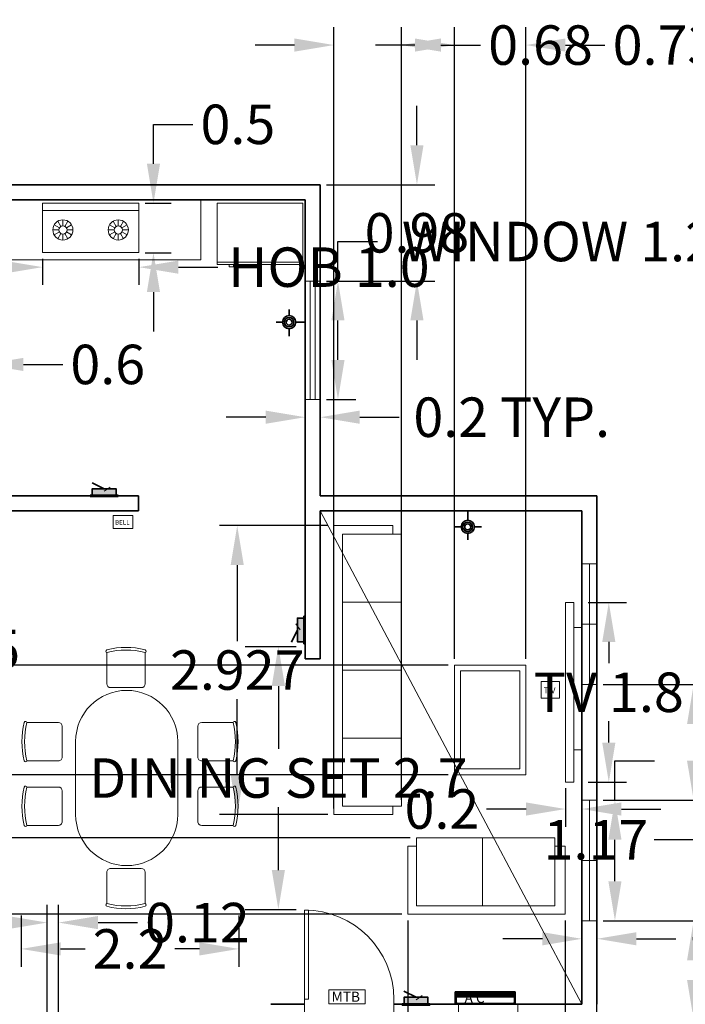
# Model space of a CAD drawing. Units: metres. Extents: x 24.2 to 58.5, y -14.5 to 15.2.
# Tile 6 of 7: x 45.2 to 51.9, y 5.2 to 15.2. Entities that reach past the tile are written whole.
import ezdxf

# ---------------------------------------------------------------- set-up
doc = ezdxf.new("R2010")
doc.units = ezdxf.units.M
doc.header["$MEASUREMENT"] = 0
for name, color, linetype, lineweight in [('A-EQPM', 163, 'Continuous', 18), ('A-FLOR', 7, 'Continuous', 25), ('A-FLOR-CASE', 163, 'Continuous', 18), ('A-GLAZ', 15, 'Continuous', 18), ('A-WALL', 7, 'Continuous', 35), ('DIMENSION', 90, 'Continuous', 18), ('DOOR', 15, 'Continuous', 18), ('E-COMM', 1, 'Continuous', 18), ('E-EQPM-LAYO', 1, 'Continuous', 13), ('E-LITE', 1, 'Continuous', 18), ('E-POWR', 1, 'Continuous', 18), ('E-POWR-EQPM', 1, 'Continuous', 18), ('Elec', 1, 'Continuous', 35), ('FURN', 163, 'Continuous', 13)]:
    doc.layers.add(name, color=color, linetype=linetype, lineweight=lineweight)
doc.styles.get("Standard").update_dxf_attribs({"font": 'arial.ttf'})
doc.dimstyles.get("Standard").update_dxf_attribs({"dimtxt": 0.4, "dimasz": 0.4, "dimexe": 0.18, "dimexo": 0.0625, "dimgap": 0.09, "dimtad": 0, "dimtih": 1, "dimtoh": 1, "dimdec": 1, "dimzin": 0, "dimdsep": 46, "dimtxsty": 'Standard', "dimcen": 0.09, "dimadec": 0, "dimazin": 0, "dimtfac": 1, "dimtdec": 1, "dimtofl": 0, "dimtmove": 0, "dimatfit": 3, "dimfxl": 1, "dimtolj": 1, "dimtzin": 0, "dimarcsym": 0})

# ---------------------------------------------------------------- blocks, each defined once
blk = doc.blocks.new('*U17')
for p, q in [((0, 0), (0, -6)), ((40, 0), (40, -6))]:
    blk.add_line(p, q)
blk.add_lwpolyline([(0, 0), (0, 40), (1.75, 40), (1.75, 0)], close=True)
blk.add_arc((0, 0), 40, 0, 90)
blk = doc.blocks.new('TV')
for points in [[(1846.64, 1133.16), (1849.49, 1133.16), (1849.49, 1073.14), (1846.64, 1073.14)], [(1846.64, 1122.37), (1844, 1122.37), (1844, 1081.48), (1846.64, 1081.48)]]:
    blk.add_lwpolyline(points, close=True)
blk = doc.blocks.new('DCHARRND')
for p, q in [((-10, -2.63815), (-10, -18.99995)), ((10, -18.99995), (10, -2.63815)), ((-8, -20.99995), (8, -20.99995))]:
    blk.add_line(p, q)
for centre, radius, start, end in [((0, -41.272), 41.272, 75.97797, 104.022), ((-9.7697, -1.94695), 0.75323, 107.8005, 188.662), ((-9.8649, -2.00005), 0.65223, 185.3119, 258.05), ((0, -42.68032), 41.272, 75.97797, 104.022), ((9.7697, -1.94695), 0.75323, 351.338, 72.19953), ((9.865, -2.00005), 0.65223, 281.95, 354.6881), ((-8, -18.99995), 2, 180, 270), ((8, -18.99995), 2, 270, 0)]:
    blk.add_arc(centre, radius, start, end)
blk = doc.blocks.new('TABLE')
for p, q in [((59.132, -4.604), (59.132, -5.611)), ((60.539, -4.604), (60.539, -5.611))]:
    blk.add_line(p, q)
for centre, start, end in [((59.836, -4.604), 0, 180), ((59.836, -5.611), 180, 0)]:
    blk.add_arc(centre, 0.704, start, end)
at = {"layer": 'FURN', "xscale": -0.0264381201488454, "yscale": 0.0264381201488454, "zscale": 0.0264381201488454}
blk.add_blockref('DCHARRND', (59.826, -3.307), dxfattribs=at)
at = {"layer": 'FURN', "yscale": 0.0264381201488454, "zscale": 0.0264381201488454}
for p, xscale, rotation in [((58.391, -4.606), -0.0264381201488454, 89.99999999999991), ((61.372, -4.606), 0.0264381201488454, 270.0000000000001), ((58.391, -5.496), -0.0264381201488454, 89.99999999999991), ((61.372, -5.496), 0.0264381201488454, 270.0000000000001), ((59.826, -6.908), 0.0264381201488454, 180)]:
    blk.add_blockref('DCHARRND', p, dxfattribs=dict(at, xscale=xscale, rotation=rotation))
blk = doc.blocks.new('*U31')
blk.add_line((0, 1), (0, -1))
blk = doc.blocks.new('*U32')
at = {"layer": 'FURN', "transparency": 16777216}
for p, rotation in [((1740.24, 1059.29), 30), ((1742.61, 1059.29), 330.0000000000001), ((1739.06, 1057.24), 90), ((1739.38, 1058.42), 59.99999999999999), ((1739.38, 1056.06), 120), ((1743.47, 1058.42), 300), ((1743.47, 1056.06), 240), ((1743.79, 1057.24), 270), ((1740.24, 1055.19), 150), ((1741.42, 1054.87), 180), ((1742.61, 1055.19), 210)]:
    blk.add_blockref('*U31', p, dxfattribs=dict(at, rotation=rotation))
blk.add_blockref('*U31', (1741.42, 1059.61), dxfattribs=at)
blk = doc.blocks.new('*U33')
blk.add_line((0, 1), (0, -1))
blk = doc.blocks.new('*U34')
at = {"layer": 'FURN', "transparency": 16777216}
for p, rotation in [((1740.24, 1059.29), 30), ((1742.61, 1059.29), 330.0000000000001), ((1739.06, 1057.24), 90), ((1739.38, 1058.42), 59.99999999999999), ((1739.38, 1056.06), 120), ((1743.47, 1058.42), 300), ((1743.47, 1056.06), 240), ((1743.79, 1057.24), 270), ((1740.24, 1055.19), 150), ((1741.42, 1054.87), 180), ((1742.61, 1055.19), 210)]:
    blk.add_blockref('*U33', p, dxfattribs=dict(at, rotation=rotation))
blk.add_blockref('*U33', (1741.42, 1059.61), dxfattribs=at)
blk = doc.blocks.new('GAS')
at = {"layer": 'FURN'}
blk.add_line((1734.58, 1063.74), (1766.85, 1063.74), dxfattribs=at)
blk.add_lwpolyline([(1734.58, 1066.15), (1766.85, 1066.15), (1766.85, 1049.65), (1734.58, 1049.65)], close=True, dxfattribs=at)
for centre, radius in [((1741.42, 1057.24), 3.37), ((1759.93, 1057.24), 3.37), ((1741.42, 1057.24), 1.37), ((1759.93, 1057.24), 1.37)]:
    blk.add_circle(centre, radius, dxfattribs=at)
for name, p in [('*U32', (0, 0)), ('*U34', (18.51, 0))]:
    blk.add_blockref(name, p, dxfattribs=at)
blk = doc.blocks.new('splight')
at = {"layer": 'Elec'}
for p, q in [((4618.17, 527.16), (4627.57, 527.16)), ((4622.87, 527.16), (4622.87, 523.87)), ((4620.58, 521.58), (4618.05, 521.58)), ((4625.16, 521.58), (4627.23, 521.58)), ((4622.87, 519.28), (4622.87, 517.03))]:
    blk.add_line(p, q, dxfattribs=at)
for radius in [2.29, 1.67, 1.04]:
    blk.add_circle((4622.87, 521.58), radius, dxfattribs=at)
blk = doc.blocks.new('WINDOW-1200')
for p, q in [((0.1529, 1.1998), (0.0005, 1.1998)), ((0.0513, -0.0002), (0.0513, 1.1998)), ((0.1021, -0.0002), (0.1021, 1.1998)), ((0.1529, -0.0002), (0.0005, -0.0002))]:
    blk.add_line(p, q)
blk = doc.blocks.new('WINDOW-1220-DIVIDED')
for p, q in [((0.1527, 1.2199), (0.0003, 1.2199)), ((0.0765, -0.0001), (0.0765, 1.2199)), ((0.1527, 0.6099), (0.0003, 0.6099)), ((0.1527, -0.0001), (0.0003, -0.0001))]:
    blk.add_line(p, q)
blk = doc.blocks.new('BELL-PLUG-POINT')
blk.add_lwpolyline([(-0.0005, 0.1301), (0.1984, 0.1301), (0.1984, 0.0005), (-0.0005, 0.0005)], close=True)
at = {"insert": (0.0191, 0.0854), "char_height": 0.04661, "attachment_point": 1}
blk.add_mtext('BELL', dxfattribs=at)
blk = doc.blocks.new('TV-POINT')
blk.add_lwpolyline([(-0.0003, 0.169), (0.1847, 0.169), (0.1847, 0.0002), (-0.0003, 0.0002)], close=True)
at = {"transparency": 33554676}
blk.add_lwpolyline([(-0.0003, 0.169), (0.1847, 0.169), (0.1847, 0.0002), (-0.0003, 0.0002)], close=True, dxfattribs=at)
at = {"insert": (0.0252, 0.1107), "char_height": 0.06075, "attachment_point": 1}
blk.add_mtext('T.V ', dxfattribs=at)
at = {"transparency": 33554676, "insert": (0.0252, 0.1107), "char_height": 0.06075, "attachment_point": 1}
blk.add_mtext('T.V ', dxfattribs=at)
blk = doc.blocks.new('METER-BOARD-TAG')
blk.add_lwpolyline([(0.0003, 0.1428), (0.3661, 0.1428), (0.3661, 0.0002), (0.0003, 0.0002)], close=True)
blk.add_text('MTB', height=0.10197).set_placement((0.0268, 0.0213))
blk = doc.blocks.new('elec box')
at = {"layer": 'Elec'}
blk.add_hatch(color=256, dxfattribs=at).paths.add_polyline_path([(3828.23, 599.29), (3828.23, 594.79), (3844.73, 594.79), (3844.73, 599.29)])
for p, q in [((3836.48, 599.29), (3828.07, 603.45)), ((3846.1, 594.79), (3826.83, 594.79)), ((3826.83, 594.79), (3826.83, 593.89)), ((3826.83, 593.89), (3846.1, 593.89)), ((3846.1, 593.89), (3846.1, 594.79))]:
    blk.add_line(p, q, dxfattribs=at)
blk.add_lwpolyline([(3828.23, 594.79), (3828.23, 599.29), (3844.73, 599.29), (3844.73, 594.79), (3828.23, 594.79)], dxfattribs=at)
blk = doc.blocks.new('SWITCHBOARD-ONE-WAY')
blk.add_line((0.1401, 0.0521), (0.201, 0.0944))
at = {"xscale": 0.0145668999005024, "yscale": 0.0145668999005024, "zscale": 0.0145668999005024}
blk.add_blockref('elec box', (-55.7455, -8.6514), dxfattribs=at)
blk = doc.blocks.new('ac')
at = {"layer": 'Elec'}
for p, q in [((12718.34, -53.78), (12674.36, -53.78)), ((12674.36, -63.02), (12674.36, -53.78)), ((12674.89, -57.52), (12717.81, -57.52)), ((12675.81, -57.52), (12675.81, -53.78)), ((12717.03, -54.85), (12675.81, -54.85)), ((12717.03, -56.21), (12675.81, -56.21)), ((12717.03, -57.52), (12717.03, -53.78)), ((12718.34, -63.02), (12718.34, -53.78)), ((12718.34, -63.02), (12674.36, -63.02))]:
    blk.add_line(p, q, dxfattribs=at)
at = {"layer": 'Elec', "ltscale": 0.1}
for p, q in [((12674.89, -61.49), (12674.89, -53.78)), ((12717.03, -54.36), (12675.81, -54.36)), ((12717.03, -55.66), (12675.81, -55.66)), ((12717.03, -56.84), (12675.81, -56.84)), ((12717.81, -61.49), (12717.81, -53.78)), ((12716.81, -62.49), (12675.89, -62.49))]:
    blk.add_line(p, q, dxfattribs=at)
at = {"layer": 'Elec'}
for centre, start, end in [((12675.89, -61.49), 180, 270), ((12716.81, -61.49), 270, 0)]:
    blk.add_arc(centre, 1, start, end, dxfattribs=at)
blk = doc.blocks.new('AC-POINT-LABELED')
at = {"xscale": 0.0137983327653967, "yscale": 0.0137983327653967, "zscale": 0.0137983327653967}
blk.add_blockref('ac', (-174.885, 0.8697), dxfattribs=at)
blk.add_text(' A C', height=0.10197).set_placement((0.0625, 0.0143))
blk = doc.blocks.new('*D59')
at = {"layer": 'Defpoints', "color": 0, "transparency": 16777216}
for p in [(48.2279, 12.5298), (48.4079, 12.5298), (48.2279, 11.3298)]:
    blk.add_point(p, dxfattribs=at)
at = {"layer": 'DIMENSION', "color": 0, "lineweight": -2, "transparency": 16777216}
for p, q in [((48.4079, 12.5298), (48.4079, 12.9298)), ((48.4079, 12.9298), (48.8079, 12.9298)), ((48.2904, 12.5298), (48.5879, 12.5298)), ((48.4079, 11.7298), (48.4079, 12.1298)), ((48.2904, 11.3298), (48.5879, 11.3298))]:
    blk.add_line(p, q, dxfattribs=at)
at = {"layer": 'DIMENSION', "color": 0, "transparency": 16777216}
for points in [[(48.3412, 12.1298), (48.4745, 12.1298), (48.4079, 12.5298)], [(48.3412, 11.7298), (48.4745, 11.7298), (48.4079, 11.3298)]]:
    blk.add_solid(points, dxfattribs=at)
at = {"layer": 'DIMENSION', "color": 0, "transparency": 16777216, "insert": (51.2608, 12.9298), "char_height": 0.4, "attachment_point": 5}
blk.add_mtext('\\A1;WINDOW 1.2 TYP.', dxfattribs=at)
blk = doc.blocks.new('*D60')
at = {"layer": 'Defpoints', "color": 0, "transparency": 16777216}
for p in [(48.0755, 11.3298), (48.2279, 11.3298), (48.2279, 11.1498)]:
    blk.add_point(p, dxfattribs=at)
at = {"layer": 'DIMENSION', "color": 0, "lineweight": -2, "transparency": 16777216}
for p, q in [((48.0755, 11.2673), (48.0755, 10.9698)), ((48.2279, 11.2673), (48.2279, 10.9698)), ((47.6755, 11.1498), (47.2755, 11.1498)), ((48.6279, 11.1498), (49.0279, 11.1498))]:
    blk.add_line(p, q, dxfattribs=at)
at = {"layer": 'DIMENSION', "color": 0, "transparency": 16777216}
for points in [[(47.6755, 11.2165), (47.6755, 11.0832), (48.0755, 11.1498)], [(48.6279, 11.2165), (48.6279, 11.0832), (48.2279, 11.1498)]]:
    blk.add_solid(points, dxfattribs=at)
at = {"layer": 'DIMENSION', "color": 0, "transparency": 16777216, "insert": (50.169, 11.1498), "char_height": 0.4, "attachment_point": 5}
blk.add_mtext('\\A1;0.2 TYP.', dxfattribs=at)
blk = doc.blocks.new('*D63')
at = {"layer": 'Defpoints', "color": 0, "transparency": 16777216}
for p in [(51.0327, 7.2681), (51.2157, 7.2681), (51.0327, 6.0481)]:
    blk.add_point(p, dxfattribs=at)
at = {"layer": 'DIMENSION', "color": 0, "lineweight": -2, "transparency": 16777216}
for p, q in [((51.2157, 7.2681), (51.2157, 7.6681)), ((51.2157, 7.6681), (51.6157, 7.6681)), ((51.0952, 7.2681), (51.3957, 7.2681)), ((51.2157, 6.4481), (51.2157, 6.8681)), ((51.0952, 6.0481), (51.3957, 6.0481))]:
    blk.add_line(p, q, dxfattribs=at)
at = {"layer": 'DIMENSION', "color": 0, "transparency": 16777216}
for points in [[(51.149, 6.8681), (51.2823, 6.8681), (51.2157, 7.2681)], [(51.149, 6.4481), (51.2823, 6.4481), (51.2157, 6.0481)]]:
    blk.add_solid(points, dxfattribs=at)
at = {"layer": 'DIMENSION', "color": 0, "transparency": 16777216, "insert": (55.2613, 7.6681), "char_height": 0.4, "attachment_point": 5}
blk.add_mtext('\\A1;DIVIDED WINDOW 1.2 TYP.', dxfattribs=at)
blk = doc.blocks.new('*D64')
at = {"layer": 'Defpoints', "color": 0, "transparency": 16777216}
for p in [(50.8803, 6.0481), (51.0327, 6.0481), (51.0327, 5.8651)]:
    blk.add_point(p, dxfattribs=at)
at = {"layer": 'DIMENSION', "color": 0, "lineweight": -2, "transparency": 16777216}
for p, q in [((50.8803, 5.9856), (50.8803, 5.6851)), ((51.0327, 5.9856), (51.0327, 5.6851)), ((50.4803, 5.8651), (50.0803, 5.8651)), ((51.4327, 5.8651), (51.8327, 5.8651))]:
    blk.add_line(p, q, dxfattribs=at)
at = {"layer": 'DIMENSION', "color": 0, "transparency": 16777216}
for points in [[(50.4803, 5.9318), (50.4803, 5.7985), (50.8803, 5.8651)], [(51.4327, 5.9318), (51.4327, 5.7985), (51.0327, 5.8651)]]:
    blk.add_solid(points, dxfattribs=at)
at = {"layer": 'DIMENSION', "color": 0, "transparency": 16777216, "insert": (52.9738, 5.8651), "char_height": 0.4, "attachment_point": 5}
blk.add_mtext('\\A1;0.2 TYP.', dxfattribs=at)
blk = doc.blocks.new('*D69')
at = {"layer": 'Defpoints', "color": 0, "transparency": 16777216}
for p in [(50.8803, 9.2728), (50.8803, 7.453), (51.1532, 7.453)]:
    blk.add_point(p, dxfattribs=at)
at = {"layer": 'DIMENSION', "color": 0, "lineweight": -2, "transparency": 16777216}
for p, q in [((50.9428, 9.2728), (51.3332, 9.2728)), ((51.1532, 8.8728), (51.1532, 8.6571)), ((51.1532, 7.853), (51.1532, 8.0686)), ((50.9428, 7.453), (51.3332, 7.453))]:
    blk.add_line(p, q, dxfattribs=at)
at = {"layer": 'DIMENSION', "color": 0, "transparency": 16777216}
for points in [[(51.0866, 8.8728), (51.2199, 8.8728), (51.1532, 9.2728)], [(51.0866, 7.853), (51.2199, 7.853), (51.1532, 7.453)]]:
    blk.add_solid(points, dxfattribs=at)
at = {"layer": 'DIMENSION', "color": 0, "transparency": 16777216, "insert": (51.1532, 8.3629), "char_height": 0.4, "attachment_point": 5}
blk.add_mtext('\\A1;TV 1.8', dxfattribs=at)
blk = doc.blocks.new('*D70')
at = {"layer": 'Defpoints', "color": 0, "transparency": 16777216}
for p in [(50.7139, 7.453), (50.8803, 7.453), (50.7139, 7.18)]:
    blk.add_point(p, dxfattribs=at)
at = {"layer": 'DIMENSION', "color": 0, "lineweight": -2, "transparency": 16777216}
for p, q in [((50.7139, 7.3905), (50.7139, 7)), ((50.8803, 7.3905), (50.8803, 7)), ((50.3139, 7.18), (49.9139, 7.18)), ((51.2803, 7.18), (51.6803, 7.18))]:
    blk.add_line(p, q, dxfattribs=at)
at = {"layer": 'DIMENSION', "color": 0, "transparency": 16777216}
for points in [[(50.3139, 7.2467), (50.3139, 7.1133), (50.7139, 7.18)], [(51.2803, 7.2467), (51.2803, 7.1133), (50.8803, 7.18)]]:
    blk.add_solid(points, dxfattribs=at)
at = {"layer": 'DIMENSION', "color": 0, "transparency": 16777216, "insert": (49.4618, 7.18), "char_height": 0.4, "attachment_point": 5}
blk.add_mtext('\\A1;0.2', dxfattribs=at)
blk = doc.blocks.new('*D74')
at = {"layer": 'Defpoints', "color": 0, "transparency": 16777216}
for p in [(43.0417, 8.8871), (43.5517, 8.8871), (43.5517, 8.7964)]:
    blk.add_point(p, dxfattribs=at)
at = {"layer": 'DIMENSION', "color": 0, "lineweight": -2, "transparency": 16777216}
for p, q in [((42.6417, 8.7964), (42.2417, 8.7964)), ((43.0417, 8.8246), (43.0417, 8.6164)), ((43.5517, 8.8246), (43.5517, 8.6164)), ((43.9517, 8.7964), (44.3517, 8.7964))]:
    blk.add_line(p, q, dxfattribs=at)
at = {"layer": 'DIMENSION', "color": 0, "transparency": 16777216}
for points in [[(42.6417, 8.863), (42.6417, 8.7297), (43.0417, 8.7964)], [(43.9517, 8.863), (43.9517, 8.7297), (43.5517, 8.7964)]]:
    blk.add_solid(points, dxfattribs=at)
at = {"layer": 'DIMENSION', "color": 0, "transparency": 16777216, "insert": (44.8074, 8.7964), "char_height": 0.4, "attachment_point": 5}
blk.add_mtext('\\A1;0.5', dxfattribs=at)
blk = doc.blocks.new('*D75')
at = {"layer": 'Defpoints', "color": 0, "transparency": 16777216}
for p in [(47.404, 8.8257), (47.8036, 8.8257), (47.404, 6.162)]:
    blk.add_point(p, dxfattribs=at)
at = {"layer": 'DIMENSION', "color": 0, "lineweight": -2, "transparency": 16777216}
for p, q in [((47.4665, 8.8257), (47.9836, 8.8257)), ((47.8036, 8.4257), (47.8036, 7.7907)), ((47.8036, 6.562), (47.8036, 7.1971)), ((47.4665, 6.162), (47.9836, 6.162))]:
    blk.add_line(p, q, dxfattribs=at)
at = {"layer": 'DIMENSION', "color": 0, "transparency": 16777216}
for points in [[(47.7369, 8.4257), (47.8702, 8.4257), (47.8036, 8.8257)], [(47.7369, 6.562), (47.8702, 6.562), (47.8036, 6.162)]]:
    blk.add_solid(points, dxfattribs=at)
at = {"layer": 'DIMENSION', "color": 0, "transparency": 16777216, "insert": (47.8036, 7.4939), "char_height": 0.4, "attachment_point": 5}
blk.add_mtext('\\A1;DINING SET 2.7', dxfattribs=at)
blk = doc.blocks.new('*D76')
at = {"layer": 'Defpoints', "color": 0, "transparency": 16777216}
for p in [(45.196, 6.162), (47.404, 6.162), (47.404, 5.7625)]:
    blk.add_point(p, dxfattribs=at)
at = {"layer": 'DIMENSION', "color": 0, "lineweight": -2, "transparency": 16777216}
for p, q in [((45.196, 6.0995), (45.196, 5.5825)), ((47.404, 6.0995), (47.404, 5.5825)), ((45.596, 5.7625), (45.8445, 5.7625)), ((47.004, 5.7625), (46.7555, 5.7625))]:
    blk.add_line(p, q, dxfattribs=at)
at = {"layer": 'DIMENSION', "color": 0, "transparency": 16777216}
for points in [[(45.596, 5.8291), (45.596, 5.6958), (45.196, 5.7625)], [(47.004, 5.8291), (47.004, 5.6958), (47.404, 5.7625)]]:
    blk.add_solid(points, dxfattribs=at)
at = {"layer": 'DIMENSION', "color": 0, "transparency": 16777216, "insert": (46.3, 5.7625), "char_height": 0.4, "attachment_point": 5}
blk.add_mtext('\\A1;2.2', dxfattribs=at)
blk = doc.blocks.new('*D77')
at = {"layer": 'Defpoints', "color": 0, "transparency": 16777216}
for p in [(45.4122, 12.817), (46.3908, 12.817), (46.3908, 12.6703)]:
    blk.add_point(p, dxfattribs=at)
at = {"layer": 'DIMENSION', "color": 0, "lineweight": -2, "transparency": 16777216}
for p, q in [((45.0122, 12.6703), (44.6122, 12.6703)), ((45.4122, 12.7545), (45.4122, 12.4903)), ((46.3908, 12.7545), (46.3908, 12.4903)), ((46.7908, 12.6703), (47.1908, 12.6703))]:
    blk.add_line(p, q, dxfattribs=at)
at = {"layer": 'DIMENSION', "color": 0, "transparency": 16777216}
for points in [[(45.0122, 12.7369), (45.0122, 12.6036), (45.4122, 12.6703)], [(46.7908, 12.7369), (46.7908, 12.6036), (46.3908, 12.6703)]]:
    blk.add_solid(points, dxfattribs=at)
at = {"layer": 'DIMENSION', "color": 0, "transparency": 16777216, "insert": (48.3165, 12.6703), "char_height": 0.4, "attachment_point": 5}
blk.add_mtext('\\A1;HOB 1.0', dxfattribs=at)
blk = doc.blocks.new('*D78')
at = {"layer": 'Defpoints', "color": 0, "transparency": 16777216}
for p in [(46.3908, 13.3173), (46.5376, 13.3173), (46.3908, 12.817)]:
    blk.add_point(p, dxfattribs=at)
at = {"layer": 'DIMENSION', "color": 0, "lineweight": -2, "transparency": 16777216}
for p, q in [((46.5376, 13.7173), (46.5376, 14.1173)), ((46.5376, 14.1173), (46.9376, 14.1173)), ((46.4533, 13.3173), (46.7176, 13.3173)), ((46.4533, 12.817), (46.7176, 12.817)), ((46.5376, 12.417), (46.5376, 12.017))]:
    blk.add_line(p, q, dxfattribs=at)
at = {"layer": 'DIMENSION', "color": 0, "transparency": 16777216}
for points in [[(46.4709, 13.7173), (46.6042, 13.7173), (46.5376, 13.3173)], [(46.4709, 12.417), (46.6042, 12.417), (46.5376, 12.817)]]:
    blk.add_solid(points, dxfattribs=at)
at = {"layer": 'DIMENSION', "color": 0, "transparency": 16777216, "insert": (47.3932, 14.1173), "char_height": 0.4, "attachment_point": 5}
blk.add_mtext('\\A1;0.5', dxfattribs=at)
blk = doc.blocks.new('*D80')
at = {"layer": 'Defpoints', "color": 0, "transparency": 16777216}
for p in [(44.2452, 11.8039), (44.82, 11.8039), (44.82, 11.6846)]:
    blk.add_point(p, dxfattribs=at)
at = {"layer": 'DIMENSION', "color": 0, "lineweight": -2, "transparency": 16777216}
for p, q in [((43.8452, 11.6846), (43.4452, 11.6846)), ((44.2452, 11.7414), (44.2452, 11.5046)), ((44.82, 11.7414), (44.82, 11.5046)), ((45.22, 11.6846), (45.62, 11.6846))]:
    blk.add_line(p, q, dxfattribs=at)
at = {"layer": 'DIMENSION', "color": 0, "transparency": 16777216}
for points in [[(43.8452, 11.7513), (43.8452, 11.6179), (44.2452, 11.6846)], [(45.22, 11.7513), (45.22, 11.6179), (44.82, 11.6846)]]:
    blk.add_solid(points, dxfattribs=at)
at = {"layer": 'DIMENSION', "color": 0, "transparency": 16777216, "insert": (46.074, 11.6846), "char_height": 0.4, "attachment_point": 5}
blk.add_mtext('\\A1;0.6', dxfattribs=at)
blk = doc.blocks.new('*D113')
at = {"layer": 'Defpoints', "color": 0, "transparency": 16777216}
for p in [(51.0327, 6.0482), (51.0327, 5.0488), (52.0132, 5.0488)]:
    blk.add_point(p, dxfattribs=at)
at = {"layer": 'DIMENSION', "color": 0, "lineweight": -2, "transparency": 16777216}
for p, q in [((51.0952, 6.0482), (52.1932, 6.0482)), ((52.0132, 5.6482), (52.0132, 5.4488)), ((51.0952, 5.0488), (52.1932, 5.0488)), ((52.0132, 5.0488), (52.0132, 4.6488)), ((52.0132, 4.6488), (51.6132, 4.6488))]:
    blk.add_line(p, q, dxfattribs=at)
at = {"layer": 'DIMENSION', "color": 0, "transparency": 16777216}
for points in [[(51.9465, 5.6482), (52.0798, 5.6482), (52.0132, 6.0482)], [(51.9465, 5.4488), (52.0798, 5.4488), (52.0132, 5.0488)]]:
    blk.add_solid(points, dxfattribs=at)
at = {"layer": 'DIMENSION', "color": 0, "transparency": 16777216, "insert": (51.0232, 4.6488), "char_height": 0.4, "attachment_point": 5}
blk.add_mtext('\\A1;1.00', dxfattribs=at)
blk = doc.blocks.new('*D114')
at = {"layer": 'Defpoints', "color": 0, "transparency": 16777216}
for p in [(51.0327, 8.4429), (51.0327, 7.2682), (52.0132, 7.2682)]:
    blk.add_point(p, dxfattribs=at)
at = {"layer": 'DIMENSION', "color": 0, "lineweight": -2, "transparency": 16777216}
for p, q in [((51.0952, 8.4429), (52.1932, 8.4429)), ((52.0132, 8.0429), (52.0132, 7.6682)), ((51.0952, 7.2682), (52.1932, 7.2682)), ((52.0132, 7.2682), (52.0132, 6.8681)), ((52.0132, 6.8681), (51.6132, 6.8681))]:
    blk.add_line(p, q, dxfattribs=at)
at = {"layer": 'DIMENSION', "color": 0, "transparency": 16777216}
for points in [[(51.9465, 8.0429), (52.0798, 8.0429), (52.0132, 8.4429)], [(51.9465, 7.6682), (52.0798, 7.6682), (52.0132, 7.2682)]]:
    blk.add_solid(points, dxfattribs=at)
at = {"layer": 'DIMENSION', "color": 0, "transparency": 16777216, "insert": (51.0225, 6.8681), "char_height": 0.4, "attachment_point": 5}
blk.add_mtext('\\A1;1.17', dxfattribs=at)
blk = doc.blocks.new('*D115')
at = {"layer": 'Defpoints', "color": 0, "transparency": 16777216}
for p in [(48.2279, 13.506), (48.2279, 12.5298), (49.2084, 12.5298)]:
    blk.add_point(p, dxfattribs=at)
at = {"layer": 'DIMENSION', "color": 0, "lineweight": -2, "transparency": 16777216}
for p, q in [((49.2084, 13.906), (49.2084, 14.306)), ((48.2904, 13.506), (49.3884, 13.506)), ((48.2904, 12.5298), (49.3884, 12.5298)), ((49.2084, 12.1298), (49.2084, 11.7298))]:
    blk.add_line(p, q, dxfattribs=at)
at = {"layer": 'DIMENSION', "color": 0, "transparency": 16777216}
for points in [[(49.1417, 13.906), (49.275, 13.906), (49.2084, 13.506)], [(49.1417, 12.1298), (49.275, 12.1298), (49.2084, 12.5298)]]:
    blk.add_solid(points, dxfattribs=at)
at = {"layer": 'DIMENSION', "color": 0, "transparency": 16777216, "insert": (49.2084, 13.0179), "char_height": 0.4, "attachment_point": 5}
blk.add_mtext('\\A1;0.98', dxfattribs=at)
blk = doc.blocks.new('*D117')
at = {"layer": 'Defpoints', "color": 0, "transparency": 16777216}
for p in [(47.3867, 10.0513), (48.3672, 10.0513), (48.3672, 7.1242)]:
    blk.add_point(p, dxfattribs=at)
at = {"layer": 'DIMENSION', "color": 0, "lineweight": -2, "transparency": 16777216}
for p, q in [((48.3047, 10.0513), (47.2067, 10.0513)), ((47.3867, 9.6513), (47.3867, 8.882)), ((47.3867, 7.5242), (47.3867, 8.2936)), ((48.3047, 7.1242), (47.2067, 7.1242))]:
    blk.add_line(p, q, dxfattribs=at)
at = {"layer": 'DIMENSION', "color": 0, "transparency": 16777216}
for points in [[(47.32, 9.6513), (47.4534, 9.6513), (47.3867, 10.0513)], [(47.32, 7.5242), (47.4534, 7.5242), (47.3867, 7.1242)]]:
    blk.add_solid(points, dxfattribs=at)
at = {"layer": 'DIMENSION', "color": 0, "transparency": 16777216, "insert": (47.3867, 8.5878), "char_height": 0.4, "attachment_point": 5}
blk.add_mtext('\\A1;2.927', dxfattribs=at)
blk = doc.blocks.new('*D118')
at = {"layer": 'Defpoints', "color": 0, "transparency": 16777216}
for p in [(49.0511, 14.9206), (49.0511, 7.2103), (48.3672, 7.1242)]:
    blk.add_point(p, dxfattribs=at)
at = {"layer": 'DIMENSION', "color": 0, "lineweight": -2, "transparency": 16777216}
for p, q in [((48.3672, 7.1867), (48.3672, 15.1006)), ((49.0511, 7.2728), (49.0511, 15.1006)), ((47.9672, 14.9206), (47.5672, 14.9206)), ((49.4511, 14.9206), (49.8511, 14.9206))]:
    blk.add_line(p, q, dxfattribs=at)
at = {"layer": 'DIMENSION', "color": 0, "transparency": 16777216}
for points in [[(47.9672, 14.9872), (47.9672, 14.8539), (48.3672, 14.9206)], [(49.4511, 14.9872), (49.4511, 14.8539), (49.0511, 14.9206)]]:
    blk.add_solid(points, dxfattribs=at)
at = {"layer": 'DIMENSION', "color": 0, "transparency": 16777216, "insert": (50.461, 14.9206), "char_height": 0.4, "attachment_point": 5}
blk.add_mtext('\\A1;0.68', dxfattribs=at)
blk = doc.blocks.new('*D119')
at = {"layer": 'Defpoints', "color": 0, "transparency": 16777216}
for p in [(49.1166, 6.114), (50.7111, 6.114), (50.7111, -0.7772)]:
    blk.add_point(p, dxfattribs=at)
at = {"layer": 'DIMENSION', "color": 0, "lineweight": -2, "transparency": 16777216}
for p, q in [((49.1166, 6.0515), (49.1166, -0.9572)), ((50.7111, 6.0515), (50.7111, -0.9572)), ((48.7166, -0.7772), (48.3166, -0.7772)), ((51.1111, -0.7772), (51.5111, -0.7772))]:
    blk.add_line(p, q, dxfattribs=at)
at = {"layer": 'DIMENSION', "color": 0, "transparency": 16777216}
for points in [[(48.7166, -0.7105), (48.7166, -0.8439), (49.1166, -0.7772)], [(51.1111, -0.7105), (51.1111, -0.8439), (50.7111, -0.7772)]]:
    blk.add_solid(points, dxfattribs=at)
at = {"layer": 'DIMENSION', "color": 0, "transparency": 16777216, "insert": (49.9138, -0.7772), "char_height": 0.4, "attachment_point": 5}
blk.add_mtext('\\A1;1.59', dxfattribs=at)
blk = doc.blocks.new('*D120')
at = {"layer": 'Defpoints', "color": 0, "transparency": 16777216}
for p in [(49.2027, 6.8888), (40.4426, 6.114), (49.1166, 6.114)]:
    blk.add_point(p, dxfattribs=at)
at = {"layer": 'DIMENSION', "color": 0, "lineweight": -2, "transparency": 16777216}
for p, q in [((40.4426, 7.2888), (40.4426, 7.6888)), ((49.1402, 6.8888), (40.2626, 6.8888)), ((49.0541, 6.114), (40.2626, 6.114)), ((40.4426, 5.714), (40.4426, 5.314))]:
    blk.add_line(p, q, dxfattribs=at)
at = {"layer": 'DIMENSION', "color": 0, "transparency": 16777216}
for points in [[(40.3759, 7.2888), (40.5092, 7.2888), (40.4426, 6.8888)], [(40.3759, 5.714), (40.5092, 5.714), (40.4426, 6.114)]]:
    blk.add_solid(points, dxfattribs=at)
at = {"layer": 'DIMENSION', "color": 0, "transparency": 16777216, "insert": (40.4426, 6.5014), "char_height": 0.4, "attachment_point": 5}
blk.add_mtext('\\A1;0.77', dxfattribs=at)
blk = doc.blocks.new('*D121')
at = {"layer": 'Defpoints', "color": 0, "transparency": 16777216}
for p in [(50.3133, 14.9206), (49.5878, 8.6391), (50.3133, 8.6391)]:
    blk.add_point(p, dxfattribs=at)
at = {"layer": 'DIMENSION', "color": 0, "lineweight": -2, "transparency": 16777216}
for p, q in [((49.5878, 8.7016), (49.5878, 15.1006)), ((50.3133, 8.7016), (50.3133, 15.1006)), ((49.1878, 14.9206), (48.7878, 14.9206)), ((50.7133, 14.9206), (51.1133, 14.9206))]:
    blk.add_line(p, q, dxfattribs=at)
at = {"layer": 'DIMENSION', "color": 0, "transparency": 16777216}
for points in [[(49.1878, 14.9872), (49.1878, 14.8539), (49.5878, 14.9206)], [(50.7133, 14.9872), (50.7133, 14.8539), (50.3133, 14.9206)]]:
    blk.add_solid(points, dxfattribs=at)
at = {"layer": 'DIMENSION', "color": 0, "transparency": 16777216, "insert": (51.7228, 14.9206), "char_height": 0.4, "attachment_point": 5}
blk.add_mtext('\\A1;0.73', dxfattribs=at)
blk = doc.blocks.new('*D122')
at = {"layer": 'Defpoints', "color": 0, "transparency": 16777216}
for p in [(49.5878, 8.6391), (40.4426, 7.5263), (49.5878, 7.5263)]:
    blk.add_point(p, dxfattribs=at)
at = {"layer": 'DIMENSION', "color": 0, "lineweight": -2, "transparency": 16777216}
for p, q in [((49.5253, 8.6391), (40.2626, 8.6391)), ((40.4426, 8.2391), (40.4426, 7.9263)), ((49.5253, 7.5263), (40.2626, 7.5263)), ((40.4426, 7.5263), (40.4426, 7.1263)), ((40.4426, 7.1263), (40.0426, 7.1263))]:
    blk.add_line(p, q, dxfattribs=at)
at = {"layer": 'DIMENSION', "color": 0, "transparency": 16777216}
for points in [[(40.3759, 8.2391), (40.5092, 8.2391), (40.4426, 8.6391)], [(40.3759, 7.9263), (40.5092, 7.9263), (40.4426, 7.5263)]]:
    blk.add_solid(points, dxfattribs=at)
at = {"layer": 'DIMENSION', "color": 0, "transparency": 16777216, "insert": (39.4905, 7.1263), "char_height": 0.4, "attachment_point": 5}
blk.add_mtext('\\A1;1.11', dxfattribs=at)
blk = doc.blocks.new('*D125')
at = {"layer": 'Defpoints', "color": 0, "transparency": 16777216}
for p in [(45.5755, 6.0293), (45.4589, 5.0488), (45.5755, 5.0488)]:
    blk.add_point(p, dxfattribs=at)
at = {"layer": 'DIMENSION', "color": 0, "lineweight": -2, "transparency": 16777216}
for p, q in [((45.4589, 5.1113), (45.4589, 6.2093)), ((45.5755, 5.1113), (45.5755, 6.2093)), ((45.0589, 6.0293), (44.6589, 6.0293)), ((45.9755, 6.0293), (46.3755, 6.0293))]:
    blk.add_line(p, q, dxfattribs=at)
at = {"layer": 'DIMENSION', "color": 0, "transparency": 16777216}
for points in [[(45.0589, 6.096), (45.0589, 5.9627), (45.4589, 6.0293)], [(45.9755, 6.096), (45.9755, 5.9627), (45.5755, 6.0293)]]:
    blk.add_solid(points, dxfattribs=at)
at = {"layer": 'DIMENSION', "color": 0, "transparency": 16777216, "insert": (46.9829, 6.0293), "char_height": 0.4, "attachment_point": 5}
blk.add_mtext('\\A1;0.12', dxfattribs=at)

msp = doc.modelspace()

# ---------------------------------------------------------------- linework, layer by layer
at = {"layer": 'A-EQPM'}
for p, q in [((47.1843, 13.3181), (47.1843, 12.6958)), ((48.0525, 13.3181), (47.1843, 13.3181)), ((48.0525, 12.6958), (48.0525, 13.3181)), ((47.1843, 12.7212), (48.0525, 12.7212)), ((47.1843, 12.6958), (48.0525, 12.6958))]:
    msp.add_line(p, q, dxfattribs=at)
msp.add_lwpolyline([(47.306, 12.6958), (47.3485, 12.6958), (47.3485, 12.6732), (47.306, 12.6732)], close=True, dxfattribs=at)
at = {"layer": 'A-FLOR'}
msp.add_line((51.0327, 1.8964), (51.0327, 5.2012), dxfattribs=at)
at = {"layer": 'A-FLOR-CASE'}
for p, q in [((47.0177, 12.7436), (47.0177, 13.3536)), ((44.8379, 12.7436), (47.0177, 12.7436))]:
    msp.add_line(p, q, dxfattribs=at)
at = {"layer": 'A-GLAZ'}
for p, q in [((49.63, 5.2012), (49.63, 5.0488)), ((50.23, 5.2012), (50.23, 5.0488))]:
    msp.add_line(p, q, dxfattribs=at)
at = {"layer": 'A-WALL'}
for p, q in [((44.0755, 13.506), (48.2279, 13.506)), ((48.2279, 10.3536), (48.2279, 13.506)), ((44.2279, 13.3536), (48.0755, 13.3536)), ((48.0755, 8.7016), (48.0755, 13.3536)), ((44.2279, 10.3536), (46.3865, 10.3536)), ((46.3865, 10.2012), (46.3865, 10.3536)), ((48.2279, 10.3536), (51.0327, 10.3536)), ((51.0327, 5.2012), (51.0327, 10.3536)), ((43.7279, 10.2012), (46.3865, 10.2012)), ((48.2279, 10.2012), (50.8803, 10.2012)), ((48.2279, 10.2012), (48.2279, 8.7016)), ((50.8803, 5.2012), (50.8803, 10.2012)), ((48.0755, 8.7016), (48.2279, 8.7016)), ((47.7279, 5.2012), (48.0698, 5.2012)), ((48.9798, 5.2012), (50.8803, 5.2012))]:
    msp.add_line(p, q, dxfattribs=at)
at = {"layer": 'E-EQPM-LAYO'}
msp.add_line((50.8803, 5.2012), (48.2279, 10.2012), dxfattribs=at)
at = {"layer": 'FURN'}
for p, q in [((49.0511, 9.2765), (48.4533, 9.2765)), ((49.0511, 8.5878), (48.4533, 8.5878)), ((49.0511, 7.8991), (48.4533, 7.8991)), ((49.8714, 6.2001), (49.8714, 6.8888)), ((50.6073, 6.2001), (50.6073, 6.8888))]:
    msp.add_line(p, q, dxfattribs=at)
for points in [[(48.965, 9.9652), (48.965, 10.0513), (48.3672, 10.0513), (48.3672, 7.1242), (48.965, 7.1242), (48.965, 7.2103)], [(50.6073, 6.8027), (50.7111, 6.8027), (50.7111, 6.114), (49.1166, 6.114), (49.1166, 6.8027), (49.2027, 6.8027)]]:
    msp.add_lwpolyline(points, dxfattribs=at)
for points in [[(48.4533, 9.9652), (48.4533, 7.2103), (49.0511, 7.2103), (49.0511, 9.9652)], [(50.3133, 7.5263), (49.5878, 7.5263), (49.5878, 8.6391), (50.3133, 8.6391)], [(50.2526, 7.5869), (49.6484, 7.5869), (49.6484, 8.5784), (50.2526, 8.5784)], [(50.6073, 6.2001), (49.2027, 6.2001), (49.2027, 6.8888), (50.6073, 6.8888)]]:
    msp.add_lwpolyline(points, close=True, dxfattribs=at)

# ---------------------------------------------------------------- block references
at = {"layer": 'A-EQPM', "xscale": 0.0303227481289544, "yscale": 0.0303227481289544, "zscale": 0.0303227481289544}
msp.add_blockref('GAS', (-7.185, -19.0112), dxfattribs=at)
at = {"layer": 'A-EQPM', "xscale": 0.0303227481289544, "yscale": 0.0303227481289544, "zscale": 0.0303227481289544, "rotation": 180}
msp.add_blockref('TV', (106.7954, 41.8134), dxfattribs=at)
at = {"layer": 'A-GLAZ'}
for name, p in [('WINDOW-1200', (48.075, 11.33)), ('WINDOW-1220-DIVIDED', (50.88, 8.443)), ('WINDOW-1220-DIVIDED', (50.88, 6.0482))]:
    msp.add_blockref(name, p, dxfattribs=at)
at = {"layer": 'DOOR', "xscale": 0.0226094875306225, "yscale": 0.0226094875306225, "zscale": 0.0226094875306225}
msp.add_blockref('*U17', (48.0698, 5.2523), dxfattribs=at)
at = {"layer": 'E-COMM'}
for name, p in [('BELL-PLUG-POINT', (46.1288, 10.0227)), ('TV-POINT', (50.4673, 8.3034))]:
    msp.add_blockref(name, p, dxfattribs=at)
at = {"layer": 'E-LITE', "xscale": -0.0291629336008972, "yscale": 0.0291629336008972, "zscale": 0.0291629336007624}
for p, rotation in [((32.702, -122.7037), 269.9999999999998), ((184.5399, -5.1723), 359.9999999999997)]:
    msp.add_blockref('splight', p, dxfattribs=dict(at, rotation=rotation))
at = {"layer": 'E-POWR'}
for name, p in [('SWITCHBOARD-ONE-WAY', (45.8979, 10.3468)), ('METER-BOARD-TAG', (48.3166, 5.2054)), ('SWITCHBOARD-ONE-WAY', (49.0588, 5.1944))]:
    msp.add_blockref(name, p, dxfattribs=at)
at = {"layer": 'E-POWR', "rotation": 90.0000000000036}
msp.add_blockref('SWITCHBOARD-ONE-WAY', (48.0752, 8.8541), dxfattribs=at)
at = {"layer": 'E-POWR-EQPM'}
msp.add_blockref('AC-POINT-LABELED', (49.5971, 5.2012), dxfattribs=at)
at = {"layer": 'FURN', "xscale": 0.7352439902187692, "yscale": 0.7352439902187692, "zscale": 0.7352439902187692}
msp.add_blockref('TABLE', (2.2723, 11.2493), dxfattribs=at)

# ---------------------------------------------------------------- dimensions: what is measured, and where the dimension line sits
at = {"layer": 'DIMENSION'}
for base, p1, p2, override, picture, middle in [((49.0511, 14.9206), (48.3672, 7.1242), (49.0511, 7.2103), {"dimdec": 2, "dimlfac": 1, "dimrnd": 0, "dimzin": 0, "dimdsep": 46, "dimlunit": 2}, '*D118', (50.461, 14.9206)), ((50.3133, 14.9206), (49.5878, 8.6391), (50.3133, 8.6391), {"dimdec": 2, "dimlfac": 1, "dimrnd": 0, "dimzin": 0, "dimdsep": 46, "dimlunit": 2}, '*D121', (51.7228, 14.9206)), ((44.82, 11.6846), (44.2452, 11.8039), (44.82, 11.8039), {"dimdec": 1, "dimlfac": 1, "dimrnd": 0, "dimzin": 0, "dimdsep": 46, "dimlunit": 2}, '*D80', (46.074, 11.6846)), ((43.5517, 8.7964), (43.0417, 8.8871), (43.5517, 8.8871), {"dimdec": 1, "dimlfac": 1, "dimrnd": 0, "dimzin": 0, "dimdsep": 46, "dimlunit": 2}, '*D74', (44.8074, 8.7964)), ((45.5755, 6.0293), (45.4589, 5.0488), (45.5755, 5.0488), {"dimdec": 2, "dimlfac": 1, "dimrnd": 0, "dimzin": 0, "dimdsep": 46, "dimlunit": 2}, '*D125', (46.9829, 6.0293)), ((47.404, 5.7625), (45.196, 6.162), (47.404, 6.162), {"dimdec": 1, "dimlfac": 1, "dimrnd": 0, "dimzin": 0, "dimdsep": 46, "dimlunit": 2}, '*D76', (46.3, 5.7625)), ((50.7111, -0.7772), (49.1166, 6.114), (50.7111, 6.114), {"dimdec": 2, "dimlfac": 1, "dimrnd": 0, "dimzin": 0, "dimdsep": 46, "dimlunit": 2}, '*D119', (49.9138, -0.7772))]:
    dim = msp.add_linear_dim(base=base, p1=p1, p2=p2, dimstyle='Standard', override=override, dxfattribs=at)
    dim.commit()
    dim.dimension.update_dxf_attribs({"geometry": picture, "text_midpoint": middle})
for base, p1, p2, angle, override, picture, middle in [((46.5376, 13.3173), (46.3908, 12.817), (46.3908, 13.3173), 90, {"dimdec": 1, "dimlfac": 1, "dimrnd": 0, "dimzin": 0, "dimdsep": 46, "dimlunit": 2}, '*D78', (47.3932, 14.1173)), ((49.2084, 12.5298), (48.2279, 13.506), (48.2279, 12.5298), 270, {"dimdec": 2, "dimlfac": 1, "dimrnd": 0, "dimzin": 0, "dimdsep": 46, "dimlunit": 2}, '*D115', (49.2084, 13.0179)), ((47.3867, 10.0513), (48.3672, 7.1242), (48.3672, 10.0513), 90, {"dimdec": 3, "dimlfac": 1, "dimrnd": 0, "dimzin": 0, "dimdsep": 46, "dimlunit": 2}, '*D117', (47.3867, 8.5878)), ((40.4426, 7.5263), (49.5878, 8.6391), (49.5878, 7.5263), 90, {"dimdec": 2, "dimlfac": 1, "dimrnd": 0, "dimzin": 0, "dimdsep": 46, "dimlunit": 2}, '*D122', (39.4905, 7.1263)), ((52.0132, 7.2681), (51.0327, 8.4429), (51.0327, 7.2681), 270, {"dimdec": 2, "dimlfac": 1, "dimrnd": 0, "dimzin": 0, "dimdsep": 46, "dimlunit": 2}, '*D114', (51.0225, 6.8681)), ((40.4426, 6.114), (49.2027, 6.8888), (49.1166, 6.114), 90, {"dimdec": 2, "dimlfac": 1, "dimrnd": 0, "dimzin": 0, "dimdsep": 46, "dimlunit": 2}, '*D120', (40.4426, 6.5014)), ((50.7139, 7.18), (50.8803, 7.453), (50.7139, 7.453), 180, {"dimdec": 1, "dimlfac": 1, "dimrnd": 0, "dimzin": 0, "dimdsep": 46, "dimlunit": 2}, '*D70', (49.4618, 7.18)), ((52.0132, 5.0488), (51.0327, 6.0481), (51.0327, 5.0488), 270, {"dimdec": 2, "dimlfac": 1, "dimrnd": 0, "dimzin": 0, "dimdsep": 46, "dimlunit": 2}, '*D113', (51.0232, 4.6488))]:
    dim = msp.add_linear_dim(base=base, p1=p1, p2=p2, angle=angle, dimstyle='Standard', override=override, dxfattribs=at)
    dim.commit()
    dim.dimension.update_dxf_attribs({"geometry": picture, "text_midpoint": middle})
for base, p1, p2, angle, text, picture, middle in [((48.4079, 12.5298), (48.2279, 11.3298), (48.2279, 12.5298), 90, 'WINDOW <> TYP.', '*D59', (51.2608, 12.9298)), ((51.1532, 7.453), (50.8803, 9.2728), (50.8803, 7.453), 270, 'TV <>', '*D69', (51.1532, 8.3629)), ((51.2157, 7.2681), (51.0327, 6.0481), (51.0327, 7.2681), 90, 'DIVIDED WINDOW <> TYP.', '*D63', (55.2613, 7.6681)), ((47.8036, 8.8257), (47.404, 6.162), (47.404, 8.8257), 90, 'DINING SET <>', '*D75', (47.8036, 7.4939))]:
    dim = msp.add_linear_dim(base=base, p1=p1, p2=p2, angle=angle, text=text, dimstyle='Standard', override={"dimdec": 1, "dimlfac": 1, "dimrnd": 0, "dimzin": 0, "dimdsep": 46, "dimlunit": 2}, dxfattribs=at)
    dim.commit()
    dim.dimension.update_dxf_attribs({"geometry": picture, "text_midpoint": middle})
for base, p1, p2, text, picture, middle in [((46.3908, 12.6703), (45.4122, 12.817), (46.3908, 12.817), 'HOB <>', '*D77', (48.3165, 12.6703)), ((48.2279, 11.1498), (48.0755, 11.3298), (48.2279, 11.3298), '<> TYP.', '*D60', (50.169, 11.1498)), ((51.0327, 5.8651), (50.8803, 6.0481), (51.0327, 6.0481), '<> TYP.', '*D64', (52.9738, 5.8651))]:
    dim = msp.add_linear_dim(base=base, p1=p1, p2=p2, text=text, dimstyle='Standard', override={"dimdec": 1, "dimlfac": 1, "dimrnd": 0, "dimzin": 0, "dimdsep": 46, "dimlunit": 2}, dxfattribs=at)
    dim.commit()
    dim.dimension.update_dxf_attribs({"geometry": picture, "text_midpoint": middle})

doc.saveas('drawing.dxf')
